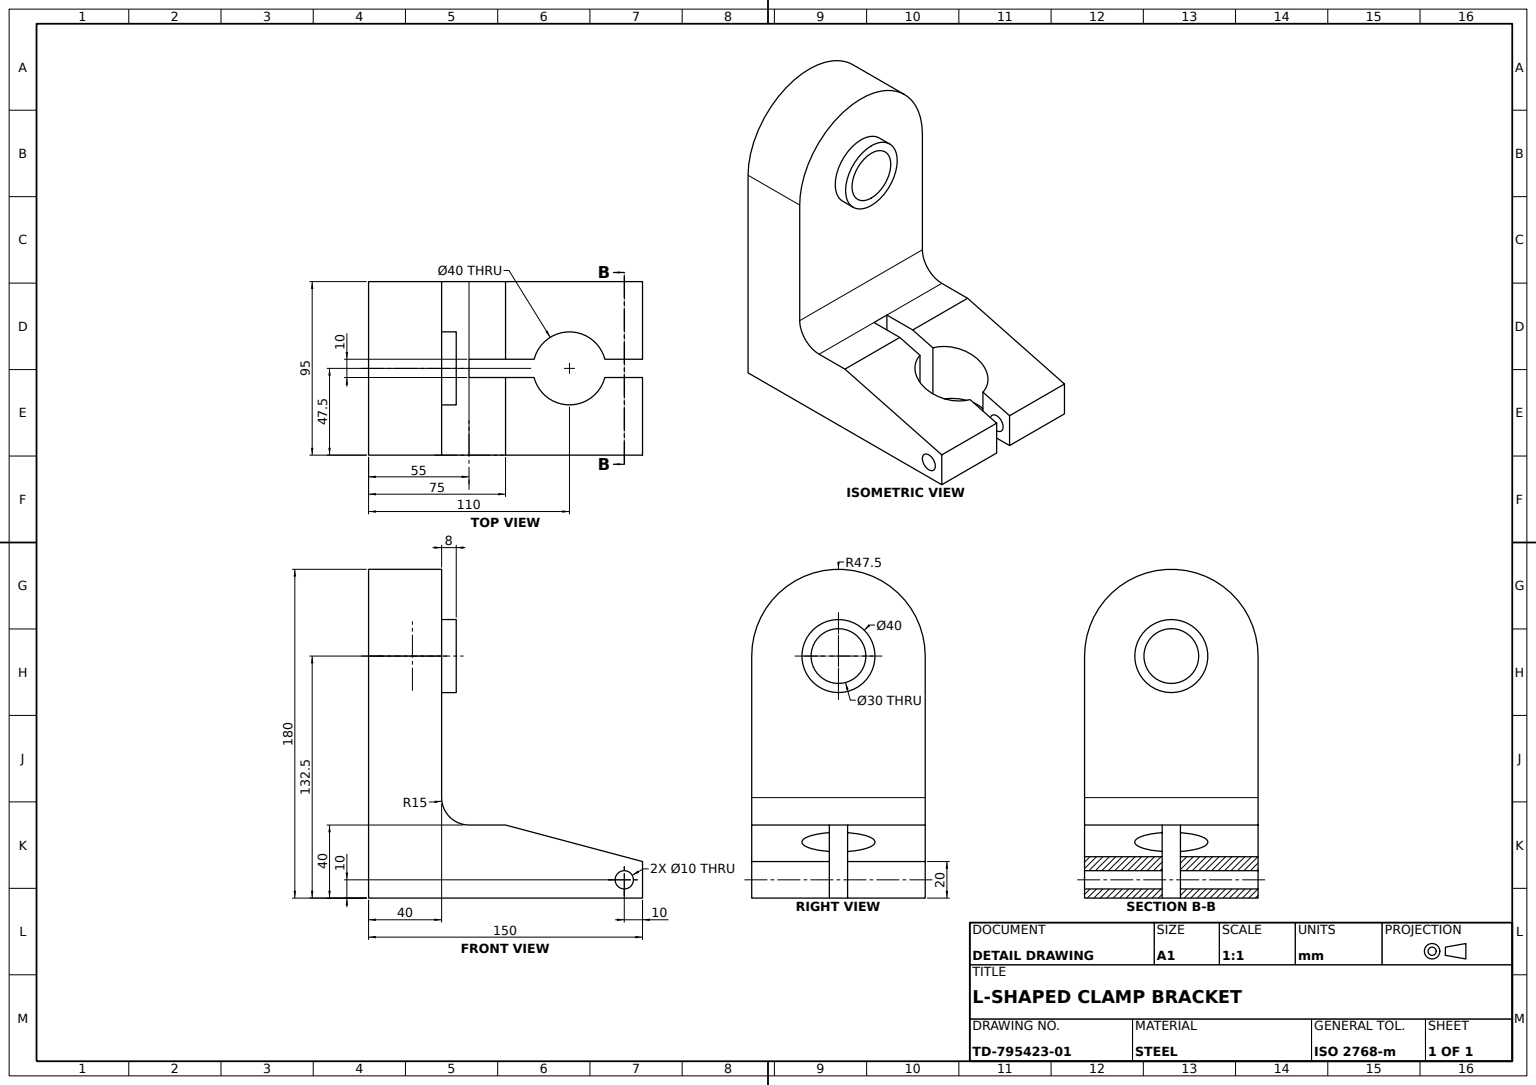
from build123d import *

# Parameters (mm, degrees)
L_BRACKET_BODY_DEPTH          = 47.5
UPRIGHT_ROUND_TOP_DEPTH       = 40
HUB_BOSS_40_SKETCH_R          = 20
HUB_BOSS_40_DEPTH             = 8
BEARING_BORE_30_SKETCH_R      = 15
BEARING_BORE_30_DEPTH         = 65
CLAMP_BORE_40_WITH_SLOT_DEPTH = 65
CLAMP_SCREW_HOLE_10_SKETCH_R  = 5
CLAMP_SCREW_HOLE_10_DEPTH     = 253.833937595


with BuildPart() as part:
    # L-Bracket Profile Sketch → L-Bracket Body (new, symmetric)
    with BuildSketch(Plane.XY):
        with BuildLine():
            Line((0, 0), (150, 0))
            Line((150, 0), (150, 20))
            Line((150, 20), (75, 40))
            Line((75, 40), (55, 40))
            ThreePointArc((55, 40), (44.393398282, 44.393398282), (40, 55))
            Line((40, 55), (40, 132.5))
            Line((40, 132.5), (0, 132.5))
            Line((0, 132.5), (0, 0))
        make_face()
    extrude(amount=L_BRACKET_BODY_DEPTH, both=True)

    # Upright Round Top Sketch → Upright Round Top (add)
    with BuildSketch(Plane.ZY):
        with BuildLine():
            Line((-47.5, 132.5), (47.5, 132.5))
            ThreePointArc((47.5, 132.5), (0, 180), (-47.5, 132.5))
        make_face()
    extrude(amount=-UPRIGHT_ROUND_TOP_DEPTH)

    # Hub Boss Ø40 Sketch → Hub Boss Ø40 (add)
    with BuildSketch(Plane(origin=(40, 0, 0), x_dir=(0, 0, -1), z_dir=(1, 0, 0))):
        with Locations(Location((0, 132.5, 0), (0, 0, 270))):
            Circle(HUB_BOSS_40_SKETCH_R)
    extrude(amount=HUB_BOSS_40_DEPTH)

    # Bearing Bore Ø30 Sketch → Bearing Bore Ø30 (cut)
    with BuildSketch(Plane(origin=(48, 0, 0), x_dir=(0, 0, -1), z_dir=(1, 0, 0))):
        with Locations(Location((0, 132.5, 0), (0, 0, 90))):
            Circle(BEARING_BORE_30_SKETCH_R)
    extrude(amount=-BEARING_BORE_30_DEPTH, mode=Mode.SUBTRACT)

    # Clamp Bore Ø40 Slot Sketch → Clamp Bore Ø40 with Slot (cut)
    with BuildSketch(Plane(origin=(0, 40, 0), x_dir=(1, 0, 0), z_dir=(0, 1, 0))):
        with BuildLine():
            Line((150, 5), (150, -5))
            Line((150, -5), (129.364916731, -5))
            ThreePointArc((129.364916731, -5), (110, -20), (90.635083269, -5))
            Line((90.635083269, -5), (55, -5))
            Line((55, -5), (55, 5))
            Line((55, 5), (90.635083269, 5))
            ThreePointArc((90.635083269, 5), (110, 20), (129.364916731, 5))
            Line((129.364916731, 5), (150, 5))
        make_face()
    extrude(amount=-CLAMP_BORE_40_WITH_SLOT_DEPTH, mode=Mode.SUBTRACT)

    # Clamp Screw Hole Ø10 Sketch → Clamp Screw Hole Ø10 (cut, through all)
    with BuildSketch(Plane.XY.offset(47.5)):
        with Locations((140, 10)):
            Circle(CLAMP_SCREW_HOLE_10_SKETCH_R)
    extrude(amount=-CLAMP_SCREW_HOLE_10_DEPTH, mode=Mode.SUBTRACT)


solid = part.part
